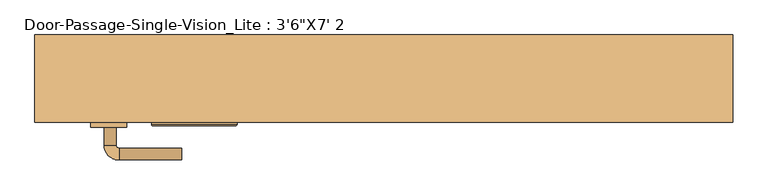
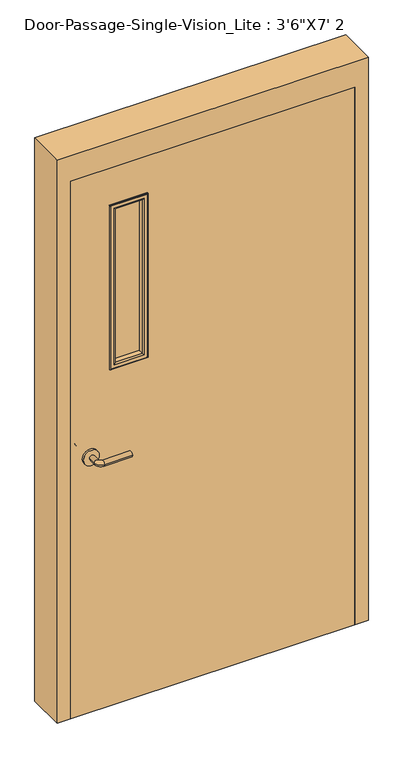
"""IFC4 building model written with IfcOpenShell, lengths in millimetres: door geometry."""

from ifc_helpers import new_model, si_unit, point, frame, frame_2d, origin, place, context, project, spatial, polyline, circle_curve, ellipse_curve, trimmed, segment, composite_curve, outline, extrude, faceted_brep, source, transform, mapped, element, save
from ifc_brep_helpers import plane_surface, cylinder_surface, revolved_surface, advanced_brep


def door_4f5842df(model_context):
    return source(origin(), model_context, "Body", "SolidModel", [
        advanced_brep(
        [(-468.390625, 14.35, 1016.0), (-448.390625, 14.35, 1016.0), (-468.390625, 44.35, 1016.0), (-448.390625, 44.35, 1016.0), (-443.390625, 49.35, 1016.0), (-443.390625, 69.35, 1016.0), (-338.390625, 69.35, 1016.0), (-338.390625, 49.35, 1016.0)],
        [
            (0, 1, circle_curve(frame((-458.390625, 14.35, 1016.0), z_axis=(0.0, -1.0, 0.0), x_axis=(1.0, 0.0, 0.0)), 10.0)),
            (1, 0, circle_curve(frame((-458.390625, 14.35, 1016.0), z_axis=(0.0, -1.0, 0.0), x_axis=(1.0, 0.0, 0.0)), 10.0)),
            (0, 2),
            (2, 3, circle_curve(frame((-458.390625, 44.35, 1016.0), z_axis=(0.0, -1.0, 0.0), x_axis=(1.0, 0.0, 0.0)), 10.0)),
            (3, 1),
            (3, 2, circle_curve(frame((-458.390625, 44.35, 1016.0), z_axis=(0.0, -1.0, 0.0), x_axis=(1.0, 0.0, 0.0)), 10.0)),
            (4, 3, circle_curve(frame((-443.390625, 44.35, 1016.0), z_axis=(0.0, 0.0, 1.0), x_axis=(-1.0, 0.0, 0.0)), 5.0)),
            (2, 5, circle_curve(frame((-443.390625, 44.35, 1016.0), z_axis=(0.0, 0.0, -1.0), x_axis=(-1.0, 0.0, 0.0)), 25.0)),
            (5, 4, circle_curve(frame((-443.390625, 59.35, 1016.0), z_axis=(-1.0, 0.0, 0.0), x_axis=(0.0, -1.0, 0.0)), 10.0)),
            (4, 5, circle_curve(frame((-443.390625, 59.35, 1016.0), z_axis=(-1.0, 0.0, 0.0), x_axis=(0.0, -1.0, 0.0)), 10.0)),
            (6, 7, circle_curve(frame((-338.390625, 59.35, 1016.0), z_axis=(1.0, 0.0, 0.0), x_axis=(0.0, -1.0, 0.0)), 10.0)),
            (7, 6, circle_curve(frame((-338.390625, 59.35, 1016.0), z_axis=(1.0, 0.0, 0.0), x_axis=(0.0, -1.0, 0.0)), 10.0)),
            (5, 6),
            (7, 4),
        ],
        [
            plane_surface(frame((-458.390625, 14.35, 1016.0), z_axis=(0.0, -1.0, 0.0), x_axis=(0.0, 0.0, 1.0))),
            cylinder_surface(frame((-458.390625, 14.35, 1016.0), z_axis=(0.0, -1.0, 0.0), x_axis=(1.0, 0.0, 0.0)), 10.0),
            revolved_surface(trimmed(ellipse_curve(frame((-458.390625, 44.35, 1016.0), z_axis=(0.0, -1.0, 0.0), x_axis=(1.0, 0.0, 0.0)), 10.0, 10.0), [point((-468.390625, 44.35, 1016.0))], [point((-448.390625, 44.35, 1016.0))], True, "CARTESIAN"), (-443.390625, 44.35, 1016.0), (0.0, 0.0, -1.0)),
            revolved_surface(trimmed(ellipse_curve(frame((-458.390625, 44.35, 1016.0), z_axis=(0.0, -1.0, 0.0), x_axis=(1.0, 0.0, 0.0)), 10.0, 10.0), [point((-448.390625, 44.35, 1016.0))], [point((-468.390625, 44.35, 1016.0))], True, "CARTESIAN"), (-443.390625, 44.35, 1016.0), (0.0, 0.0, -1.0)),
            plane_surface(frame((-338.390625, 59.35, 1016.0), z_axis=(1.0, 0.0, 0.0), x_axis=(0.0, 0.0, 1.0))),
            cylinder_surface(frame((-443.390625, 59.35, 1016.0), z_axis=(-1.0, 0.0, 0.0), x_axis=(0.0, -1.0, 0.0)), 10.0),
        ],
        [
            (0, [[1, 2]]),
            (1, [[-1, 3, 4, 5]]),
            (1, [[-2, -5, 6, -3]]),
            (2, [[7, -4, 8, 9]]),
            (3, [[-8, -6, -7, 10]]),
            (4, [[11, 12]]),
            (5, [[-9, 13, -12, 14]]),
            (5, [[-10, -14, -11, -13]]),
        ],
    ),
        extrude(outline(composite_curve([segment(trimmed(circle_curve(frame_2d((1016.0, -460.890625)), 30.0), [point((1016.0, -490.890625))], [point((1016.0, -430.890625))], False, "CARTESIAN"), True, "CONTINUOUS"), segment(trimmed(circle_curve(frame_2d((1016.0, -460.890625)), 30.0), [point((1016.0, -430.890625))], [point((1016.0, -490.890625))], False, "CARTESIAN"), True, "CONTINUOUS")], self_intersect=False)), frame((0.0, 6.35, 0.0), z_axis=(0.0, 1.0, 0.0), x_axis=(0.0, 0.0, 1.0)), (0.0, 0.0, 1.0), 8.0),
        advanced_brep(
        [(-468.390625, -46.1, 1016.0), (-448.390625, -46.1, 1016.0), (-448.390625, -76.1, 1016.0), (-468.390625, -76.1, 1016.0), (-443.390625, -81.1, 1016.0), (-443.390625, -101.1, 1016.0), (-338.390625, -101.1, 1016.0), (-338.390625, -81.1, 1016.0)],
        [
            (0, 1, circle_curve(frame((-458.390625, -46.1, 1016.0), z_axis=(0.0, 1.0, 0.0), x_axis=(1.0, 0.0, 0.0)), 10.0)),
            (1, 0, circle_curve(frame((-458.390625, -46.1, 1016.0), z_axis=(0.0, 1.0, 0.0), x_axis=(1.0, 0.0, 0.0)), 10.0)),
            (1, 2),
            (2, 3, circle_curve(frame((-458.390625, -76.1, 1016.0), z_axis=(0.0, 1.0, 0.0), x_axis=(1.0, 0.0, 0.0)), 10.0)),
            (3, 0),
            (3, 2, circle_curve(frame((-458.390625, -76.1, 1016.0), z_axis=(0.0, 1.0, 0.0), x_axis=(1.0, 0.0, 0.0)), 10.0)),
            (4, 5, circle_curve(frame((-443.390625, -91.1, 1016.0), z_axis=(-1.0, 0.0, 0.0), x_axis=(0.0, 1.0, 0.0)), 10.0)),
            (5, 3, circle_curve(frame((-443.390625, -76.1, 1016.0), z_axis=(0.0, 0.0, -1.0), x_axis=(-1.0, 0.0, 0.0)), 25.0)),
            (2, 4, circle_curve(frame((-443.390625, -76.1, 1016.0), z_axis=(0.0, 0.0, 1.0), x_axis=(-1.0, 0.0, 0.0)), 5.0)),
            (5, 4, circle_curve(frame((-443.390625, -91.1, 1016.0), z_axis=(-1.0, 0.0, 0.0), x_axis=(0.0, 1.0, 0.0)), 10.0)),
            (6, 7, circle_curve(frame((-338.390625, -91.1, 1016.0), z_axis=(1.0, 0.0, 0.0), x_axis=(0.0, 1.0, 0.0)), 10.0)),
            (7, 6, circle_curve(frame((-338.390625, -91.1, 1016.0), z_axis=(1.0, 0.0, 0.0), x_axis=(0.0, 1.0, 0.0)), 10.0)),
            (4, 7),
            (6, 5),
        ],
        [
            plane_surface(frame((-458.390625, -46.1, 1016.0), z_axis=(0.0, 1.0, 0.0), x_axis=(0.0, 0.0, 1.0))),
            cylinder_surface(frame((-458.390625, -46.1, 1016.0), z_axis=(0.0, 1.0, 0.0), x_axis=(1.0, 0.0, 0.0)), 10.0),
            revolved_surface(trimmed(ellipse_curve(frame((-458.390625, -76.1, 1016.0), z_axis=(0.0, -1.0, 0.0), x_axis=(1.0, 0.0, 0.0)), 10.0, 10.0), [point((-468.390625, -76.1, 1016.0))], [point((-448.390625, -76.1, 1016.0))], True, "CARTESIAN"), (-443.390625, -76.1, 1016.0), (0.0, 0.0, -1.0)),
            revolved_surface(trimmed(ellipse_curve(frame((-458.390625, -76.1, 1016.0), z_axis=(0.0, -1.0, 0.0), x_axis=(1.0, 0.0, 0.0)), 10.0, 10.0), [point((-448.390625, -76.1, 1016.0))], [point((-468.390625, -76.1, 1016.0))], True, "CARTESIAN"), (-443.390625, -76.1, 1016.0), (0.0, 0.0, -1.0)),
            plane_surface(frame((-338.390625, -91.1, 1016.0), z_axis=(1.0, 0.0, 0.0), x_axis=(0.0, 0.0, 1.0))),
            cylinder_surface(frame((-443.390625, -91.1, 1016.0), z_axis=(-1.0, 0.0, 0.0), x_axis=(0.0, 1.0, 0.0)), 10.0),
        ],
        [
            (0, [[1, 2]]),
            (1, [[3, 4, 5, -2]]),
            (1, [[-5, 6, -3, -1]]),
            (2, [[7, 8, -4, 9]]),
            (3, [[10, -9, -6, -8]]),
            (4, [[11, 12]]),
            (5, [[13, -11, 14, -7]]),
            (5, [[-14, -12, -13, -10]]),
        ],
    ),
        extrude(outline(composite_curve([segment(trimmed(circle_curve(frame_2d((1016.0, -460.890625)), 30.0), [point((1016.0, -490.890625))], [point((1016.0, -430.890625))], False, "CARTESIAN"), True, "CONTINUOUS"), segment(trimmed(circle_curve(frame_2d((1016.0, -460.890625)), 30.0), [point((1016.0, -430.890625))], [point((1016.0, -490.890625))], False, "CARTESIAN"), True, "CONTINUOUS")], self_intersect=False)), frame((0.0, -46.1, 0.0), z_axis=(0.0, 1.0, 0.0), x_axis=(0.0, 0.0, 1.0)), (0.0, 0.0, 1.0), 8.0),
        extrude(outline(polyline([(2133.6, -533.4), (0.0, -533.4), (0.0, 533.4), (2133.6, 533.4), (2133.6, -533.4)]), holes=[polyline([(1981.2, -381.0), (1981.2, -254.0), (1346.2, -254.0), (1346.2, -381.0), (1981.2, -381.0)])]), frame((0.0, -38.1, 0.0), z_axis=(0.0, 1.0, 0.0), x_axis=(0.0, 0.0, 1.0)), (0.0, 0.0, 1.0), 44.45),
        faceted_brep([(533.4, 11.1125, 0.0), (517.525, 11.1125, 0.0), (517.525, 58.7375, 0.0), (533.4, 58.7375, 0.0), (533.4, 107.95, 0.0), (584.2, 107.95, 0.0), (584.2, -38.1, 0.0), (533.4, -38.1, 0.0), (533.4, -38.1, 2133.6), (533.4, 11.1125, 2133.6), (584.2, -38.1, 2235.2), (-584.2, -38.1, 2235.2), (-584.2, -38.1, 0.0), (-533.4, -38.1, 0.0), (-533.4, -38.1, 2133.6), (584.2, 107.95, 2235.2), (533.4, 107.95, 2133.6), (-533.4, 107.95, 2133.6), (-533.4, 107.95, 0.0), (-584.2, 107.95, 0.0), (-584.2, 107.95, 2235.2), (533.4, 58.7375, 2133.6), (517.525, 58.7375, 2117.725), (-517.525, 58.7375, 2117.725), (-517.525, 58.7375, 0.0), (-533.4, 58.7375, 0.0), (-533.4, 58.7375, 2133.6), (517.525, 11.1125, 2117.725), (-533.4, 11.1125, 2133.6), (-533.4, 11.1125, 0.0), (-517.525, 11.1125, 0.0), (-517.525, 11.1125, 2117.725)], [[[0, 1, 2, 3, 4, 5, 6, 7]], [[7, 8, 9, 0]], [[6, 10, 11, 12, 13, 14, 8, 7]], [[5, 15, 10, 6]], [[4, 16, 17, 18, 19, 20, 15, 5]], [[3, 21, 16, 4]], [[2, 22, 23, 24, 25, 26, 21, 3]], [[1, 27, 22, 2]], [[0, 9, 28, 29, 30, 31, 27, 1]], [[8, 14, 28, 9]], [[16, 21, 26, 17]], [[22, 27, 31, 23]], [[12, 19, 18, 25, 24, 30, 29, 13]], [[13, 29, 28, 14]], [[11, 20, 19, 12]], [[17, 26, 25, 18]], [[23, 31, 30, 24]], [[15, 20, 11, 10]]]),
        extrude(outline(polyline([(-254.0, -12.7), (-254.0, -19.05), (-381.0, -19.05), (-381.0, -12.7), (-254.0, -12.7)])), frame((0.0, 0.0, 1346.2), z_axis=(0.0, 0.0, 1.0), x_axis=(1.0, 0.0, 0.0)), (0.0, 0.0, 1.0), 635.0),
        advanced_brep(
        [(-381.0, -19.05, 1981.2), (-381.0, -19.05, 1346.2), (-381.0, -38.1, 1346.2), (-381.0, -38.1, 1981.2), (-369.0, -39.1, 1969.2), (-369.0, -39.1, 1358.2), (-369.0, -19.05, 1358.2), (-369.0, -19.05, 1969.2), (-374.0, -44.1, 1974.2), (-374.0, -44.1, 1353.2), (-389.0, -42.1, 1989.2), (-389.0, -42.1, 1338.2), (-387.0, -44.1, 1340.2), (-387.0, -44.1, 1987.2), (-389.0, -38.1, 1989.2), (-389.0, -38.1, 1338.2), (-254.0, -19.05, 1346.2), (-254.0, -38.1, 1346.2), (-266.0, -39.1, 1358.2), (-266.0, -19.05, 1358.2), (-261.0, -44.1, 1353.2), (-246.0, -42.1, 1338.2), (-248.0, -44.1, 1340.2), (-246.0, -38.1, 1338.2), (-254.0, -19.05, 1981.2), (-254.0, -38.1, 1981.2), (-266.0, -39.1, 1969.2), (-266.0, -19.05, 1969.2), (-261.0, -44.1, 1974.2), (-246.0, -42.1, 1989.2), (-248.0, -44.1, 1987.2), (-246.0, -38.1, 1989.2)],
        [
            (0, 1),
            (1, 2),
            (2, 3),
            (3, 0),
            (4, 5),
            (5, 6),
            (6, 7),
            (7, 4),
            (8, 9),
            (9, 5, ellipse_curve(frame((-374.0, -39.1, 1353.2), z_axis=(-0.7071067811865475, 0.0, 0.7071067811865475), x_axis=(0.7071067811865474, 0.0, 0.7071067811865476)), 7.0710678, 5.0)),
            (4, 8, ellipse_curve(frame((-374.0, -39.1, 1974.2), z_axis=(-0.7071067811865475, 0.0, -0.7071067811865475), x_axis=(-0.7071067811865474, 0.0, 0.7071067811865476)), 7.0710678, 5.0)),
            (10, 11),
            (11, 12, ellipse_curve(frame((-387.0, -42.1, 1340.2), z_axis=(-0.7071067811865475, 0.0, 0.7071067811865475), x_axis=(0.7071067811865474, 0.0, 0.7071067811865476)), 2.8284271, 2.0)),
            (12, 13),
            (13, 10, ellipse_curve(frame((-387.0, -42.1, 1987.2), z_axis=(-0.7071067811865475, 0.0, -0.7071067811865475), x_axis=(-0.7071067811865474, 0.0, 0.7071067811865476)), 2.8284271, 2.0)),
            (14, 15),
            (15, 11),
            (10, 14),
            (1, 16),
            (16, 17),
            (17, 2),
            (5, 18),
            (18, 19),
            (19, 6),
            (9, 20),
            (20, 18, ellipse_curve(frame((-261.0, -39.1, 1353.2), z_axis=(-0.7071067811865475, 0.0, -0.7071067811865475), x_axis=(-0.7071067811865476, 0.0, 0.7071067811865474)), 7.0710678, 5.0)),
            (11, 21),
            (21, 22, ellipse_curve(frame((-248.0, -42.1, 1340.2), z_axis=(-0.7071067811865475, 0.0, -0.7071067811865475), x_axis=(-0.7071067811865476, 0.0, 0.7071067811865474)), 2.8284271, 2.0)),
            (22, 12),
            (15, 23),
            (23, 21),
            (16, 24),
            (24, 25),
            (25, 17),
            (18, 26),
            (26, 27),
            (27, 19),
            (20, 28),
            (28, 26, ellipse_curve(frame((-261.0, -39.1, 1974.2), z_axis=(0.7071067811865475, 0.0, -0.7071067811865475), x_axis=(-0.7071067811865474, 0.0, -0.7071067811865476)), 7.0710678, 5.0)),
            (21, 29),
            (29, 30, ellipse_curve(frame((-248.0, -42.1, 1987.2), z_axis=(0.7071067811865475, 0.0, -0.7071067811865475), x_axis=(-0.7071067811865474, 0.0, -0.7071067811865476)), 2.8284271, 2.0)),
            (30, 22),
            (23, 31),
            (31, 29),
            (14, 31),
            (25, 3),
            (24, 0),
            (27, 7),
            (26, 4),
            (28, 8),
            (30, 13),
            (29, 10),
        ],
        [
            plane_surface(frame((-381.0, -38.1, 1981.2), z_axis=(-1.0, 0.0, 0.0), x_axis=(0.0, 0.0, -1.0))),
            plane_surface(frame((-369.0, -19.05, 1969.2), z_axis=(1.0, 0.0, 0.0), x_axis=(0.0, 0.0, -1.0))),
            cylinder_surface(frame((-374.0, -39.1, 1981.2), z_axis=(0.0, 0.0, 1.0), x_axis=(-1.0, 0.0, 0.0)), 5.0),
            cylinder_surface(frame((-387.0, -42.1, 1981.2), z_axis=(0.0, 0.0, 1.0), x_axis=(-1.0, 0.0, 0.0)), 2.0),
            plane_surface(frame((-389.0, -42.1, 1989.2), z_axis=(-1.0, 0.0, 0.0), x_axis=(0.0, 0.0, -1.0))),
            plane_surface(frame((-381.0, -38.1, 1346.2), z_axis=(0.0, 0.0, -1.0), x_axis=(1.0, 0.0, 0.0))),
            plane_surface(frame((-369.0, -19.05, 1358.2), z_axis=(0.0, 0.0, 1.0), x_axis=(1.0, 0.0, 0.0))),
            cylinder_surface(frame((-381.0, -39.1, 1353.2), z_axis=(-1.0, 0.0, 0.0), x_axis=(0.0, 0.0, -1.0)), 5.0),
            cylinder_surface(frame((-381.0, -42.1, 1340.2), z_axis=(-1.0, 0.0, 0.0), x_axis=(0.0, 0.0, -1.0)), 2.0),
            plane_surface(frame((-389.0, -42.1, 1338.2), z_axis=(0.0, 0.0, -1.0), x_axis=(1.0, 0.0, 0.0))),
            plane_surface(frame((-254.0, -38.1, 1346.2), z_axis=(1.0, 0.0, 0.0), x_axis=(0.0, 0.0, 1.0))),
            plane_surface(frame((-266.0, -19.05, 1358.2), z_axis=(-1.0, 0.0, 0.0), x_axis=(0.0, 0.0, 1.0))),
            cylinder_surface(frame((-261.0, -39.1, 1346.2), z_axis=(0.0, 0.0, -1.0), x_axis=(1.0, 0.0, 0.0)), 5.0),
            cylinder_surface(frame((-248.0, -42.1, 1346.2), z_axis=(0.0, 0.0, -1.0), x_axis=(1.0, 0.0, 0.0)), 2.0),
            plane_surface(frame((-246.0, -42.1, 1338.2), z_axis=(1.0, 0.0, 0.0), x_axis=(0.0, 0.0, 1.0))),
            plane_surface(frame((-246.0, -38.1, 1989.2), z_axis=(0.0, 1.0, 0.0), x_axis=(-1.0, 0.0, 0.0))),
            plane_surface(frame((-254.0, -38.1, 1981.2), z_axis=(0.0, 0.0, 1.0), x_axis=(-1.0, 0.0, 0.0))),
            plane_surface(frame((-254.0, -19.05, 1981.2), z_axis=(0.0, 1.0, 0.0), x_axis=(-1.0, 0.0, 0.0))),
            plane_surface(frame((-266.0, -19.05, 1969.2), z_axis=(0.0, 0.0, -1.0), x_axis=(-1.0, 0.0, 0.0))),
            cylinder_surface(frame((-254.0, -39.1, 1974.2), z_axis=(1.0, 0.0, 0.0), x_axis=(0.0, 0.0, 1.0)), 5.0),
            plane_surface(frame((-261.0, -44.1, 1974.2), z_axis=(0.0, -1.0, 0.0), x_axis=(-1.0, 0.0, 0.0))),
            cylinder_surface(frame((-254.0, -42.1, 1987.2), z_axis=(1.0, 0.0, 0.0), x_axis=(0.0, 0.0, 1.0)), 2.0),
            plane_surface(frame((-246.0, -42.1, 1989.2), z_axis=(0.0, 0.0, 1.0), x_axis=(-1.0, 0.0, 0.0))),
        ],
        [
            (0, [[1, 2, 3, 4]]),
            (1, [[5, 6, 7, 8]]),
            (2, [[9, 10, -5, 11]]),
            (3, [[12, 13, 14, 15]]),
            (4, [[16, 17, -12, 18]]),
            (5, [[19, 20, 21, -2]]),
            (6, [[22, 23, 24, -6]]),
            (7, [[25, 26, -22, -10]]),
            (8, [[27, 28, 29, -13]]),
            (9, [[30, 31, -27, -17]]),
            (10, [[32, 33, 34, -20]]),
            (11, [[35, 36, 37, -23]]),
            (12, [[38, 39, -35, -26]]),
            (13, [[40, 41, 42, -28]]),
            (14, [[43, 44, -40, -31]]),
            (15, [[-16, 45, -43, -30], [-3, -21, -34, 46]]),
            (16, [[47, -4, -46, -33]]),
            (17, [[-1, -47, -32, -19], [-7, -24, -37, 48]]),
            (18, [[49, -8, -48, -36]]),
            (19, [[50, -11, -49, -39]]),
            (20, [[-14, -29, -42, 51], [-9, -50, -38, -25]]),
            (21, [[52, -15, -51, -41]]),
            (22, [[-45, -18, -52, -44]]),
        ],
    ),
        advanced_brep(
        [(-381.0, -12.7, 1346.2), (-381.0, -12.7, 1981.2), (-381.0, 6.35, 1981.2), (-381.0, 6.35, 1346.2), (-369.0, 7.35, 1358.2), (-369.0, 7.35, 1969.2), (-369.0, -12.7, 1969.2), (-369.0, -12.7, 1358.2), (-374.0, 12.35, 1353.2), (-374.0, 12.35, 1974.2), (-389.0, 10.35, 1338.2), (-389.0, 10.35, 1989.2), (-387.0, 12.35, 1987.2), (-387.0, 12.35, 1340.2), (-389.0, 6.35, 1338.2), (-389.0, 6.35, 1989.2), (-254.0, -12.7, 1981.2), (-254.0, 6.35, 1981.2), (-266.0, 7.35, 1969.2), (-266.0, -12.7, 1969.2), (-261.0, 12.35, 1974.2), (-246.0, 10.35, 1989.2), (-248.0, 12.35, 1987.2), (-246.0, 6.35, 1989.2), (-254.0, -12.7, 1346.2), (-254.0, 6.35, 1346.2), (-266.0, 7.35, 1358.2), (-266.0, -12.7, 1358.2), (-261.0, 12.35, 1353.2), (-246.0, 10.35, 1338.2), (-248.0, 12.35, 1340.2), (-246.0, 6.35, 1338.2)],
        [
            (0, 1),
            (1, 2),
            (2, 3),
            (3, 0),
            (4, 5),
            (5, 6),
            (6, 7),
            (7, 4),
            (8, 9),
            (9, 5, ellipse_curve(frame((-374.0, 7.35, 1974.2), z_axis=(-0.7071067811865475, 0.0, -0.7071067811865475), x_axis=(0.7071067811865474, 0.0, -0.7071067811865476)), 7.0710678, 5.0)),
            (4, 8, ellipse_curve(frame((-374.0, 7.35, 1353.2), z_axis=(-0.7071067811865475, 0.0, 0.7071067811865475), x_axis=(-0.7071067811865474, 0.0, -0.7071067811865476)), 7.0710678, 5.0)),
            (10, 11),
            (11, 12, ellipse_curve(frame((-387.0, 10.35, 1987.2), z_axis=(-0.7071067811865475, 0.0, -0.7071067811865475), x_axis=(0.7071067811865474, 0.0, -0.7071067811865476)), 2.8284271, 2.0)),
            (12, 13),
            (13, 10, ellipse_curve(frame((-387.0, 10.35, 1340.2), z_axis=(-0.7071067811865475, 0.0, 0.7071067811865475), x_axis=(-0.7071067811865474, 0.0, -0.7071067811865476)), 2.8284271, 2.0)),
            (14, 15),
            (15, 11),
            (10, 14),
            (1, 16),
            (16, 17),
            (17, 2),
            (5, 18),
            (18, 19),
            (19, 6),
            (9, 20),
            (20, 18, ellipse_curve(frame((-261.0, 7.35, 1974.2), z_axis=(-0.7071067811865475, 0.0, 0.7071067811865475), x_axis=(-0.7071067811865476, 0.0, -0.7071067811865474)), 7.0710678, 5.0)),
            (11, 21),
            (21, 22, ellipse_curve(frame((-248.0, 10.35, 1987.2), z_axis=(-0.7071067811865475, 0.0, 0.7071067811865475), x_axis=(-0.7071067811865476, 0.0, -0.7071067811865474)), 2.8284271, 2.0)),
            (22, 12),
            (15, 23),
            (23, 21),
            (16, 24),
            (24, 25),
            (25, 17),
            (18, 26),
            (26, 27),
            (27, 19),
            (20, 28),
            (28, 26, ellipse_curve(frame((-261.0, 7.35, 1353.2), z_axis=(0.7071067811865475, 0.0, 0.7071067811865475), x_axis=(-0.7071067811865474, 0.0, 0.7071067811865476)), 7.0710678, 5.0)),
            (21, 29),
            (29, 30, ellipse_curve(frame((-248.0, 10.35, 1340.2), z_axis=(0.7071067811865475, 0.0, 0.7071067811865475), x_axis=(-0.7071067811865474, 0.0, 0.7071067811865476)), 2.8284271, 2.0)),
            (30, 22),
            (23, 31),
            (31, 29),
            (14, 31),
            (25, 3),
            (24, 0),
            (27, 7),
            (26, 4),
            (28, 8),
            (30, 13),
            (29, 10),
        ],
        [
            plane_surface(frame((-381.0, 6.35, 1346.2), z_axis=(-1.0, 0.0, 0.0), x_axis=(0.0, 0.0, 1.0))),
            plane_surface(frame((-369.0, -12.7, 1358.2), z_axis=(1.0, 0.0, 0.0), x_axis=(0.0, 0.0, 1.0))),
            cylinder_surface(frame((-374.0, 7.35, 1346.2), z_axis=(0.0, 0.0, -1.0), x_axis=(-1.0, 0.0, 0.0)), 5.0),
            cylinder_surface(frame((-387.0, 10.35, 1346.2), z_axis=(0.0, 0.0, -1.0), x_axis=(-1.0, 0.0, 0.0)), 2.0),
            plane_surface(frame((-389.0, 10.35, 1338.2), z_axis=(-1.0, 0.0, 0.0), x_axis=(0.0, 0.0, 1.0))),
            plane_surface(frame((-381.0, 6.35, 1981.2), z_axis=(0.0, 0.0, 1.0), x_axis=(1.0, 0.0, 0.0))),
            plane_surface(frame((-369.0, -12.7, 1969.2), z_axis=(0.0, 0.0, -1.0), x_axis=(1.0, 0.0, 0.0))),
            cylinder_surface(frame((-381.0, 7.35, 1974.2), z_axis=(-1.0, 0.0, 0.0), x_axis=(0.0, 0.0, 1.0)), 5.0),
            cylinder_surface(frame((-381.0, 10.35, 1987.2), z_axis=(-1.0, 0.0, 0.0), x_axis=(0.0, 0.0, 1.0)), 2.0),
            plane_surface(frame((-389.0, 10.35, 1989.2), z_axis=(0.0, 0.0, 1.0), x_axis=(1.0, 0.0, 0.0))),
            plane_surface(frame((-254.0, 6.35, 1981.2), z_axis=(1.0, 0.0, 0.0), x_axis=(0.0, 0.0, -1.0))),
            plane_surface(frame((-266.0, -12.7, 1969.2), z_axis=(-1.0, 0.0, 0.0), x_axis=(0.0, 0.0, -1.0))),
            cylinder_surface(frame((-261.0, 7.35, 1981.2), z_axis=(0.0, 0.0, 1.0), x_axis=(1.0, 0.0, 0.0)), 5.0),
            cylinder_surface(frame((-248.0, 10.35, 1981.2), z_axis=(0.0, 0.0, 1.0), x_axis=(1.0, 0.0, 0.0)), 2.0),
            plane_surface(frame((-246.0, 10.35, 1989.2), z_axis=(1.0, 0.0, 0.0), x_axis=(0.0, 0.0, -1.0))),
            plane_surface(frame((-246.0, 6.35, 1338.2), z_axis=(0.0, -1.0, 0.0), x_axis=(-1.0, 0.0, 0.0))),
            plane_surface(frame((-254.0, 6.35, 1346.2), z_axis=(0.0, 0.0, -1.0), x_axis=(-1.0, 0.0, 0.0))),
            plane_surface(frame((-254.0, -12.7, 1346.2), z_axis=(0.0, -1.0, 0.0), x_axis=(-1.0, 0.0, 0.0))),
            plane_surface(frame((-266.0, -12.7, 1358.2), z_axis=(0.0, 0.0, 1.0), x_axis=(-1.0, 0.0, 0.0))),
            cylinder_surface(frame((-254.0, 7.35, 1353.2), z_axis=(1.0, 0.0, 0.0), x_axis=(0.0, 0.0, -1.0)), 5.0),
            plane_surface(frame((-261.0, 12.35, 1353.2), z_axis=(0.0, 1.0, 0.0), x_axis=(-1.0, 0.0, 0.0))),
            cylinder_surface(frame((-254.0, 10.35, 1340.2), z_axis=(1.0, 0.0, 0.0), x_axis=(0.0, 0.0, -1.0)), 2.0),
            plane_surface(frame((-246.0, 10.35, 1338.2), z_axis=(0.0, 0.0, -1.0), x_axis=(-1.0, 0.0, 0.0))),
        ],
        [
            (0, [[1, 2, 3, 4]]),
            (1, [[5, 6, 7, 8]]),
            (2, [[9, 10, -5, 11]]),
            (3, [[12, 13, 14, 15]]),
            (4, [[16, 17, -12, 18]]),
            (5, [[19, 20, 21, -2]]),
            (6, [[22, 23, 24, -6]]),
            (7, [[25, 26, -22, -10]]),
            (8, [[27, 28, 29, -13]]),
            (9, [[30, 31, -27, -17]]),
            (10, [[32, 33, 34, -20]]),
            (11, [[35, 36, 37, -23]]),
            (12, [[38, 39, -35, -26]]),
            (13, [[40, 41, 42, -28]]),
            (14, [[43, 44, -40, -31]]),
            (15, [[-16, 45, -43, -30], [-3, -21, -34, 46]]),
            (16, [[47, -4, -46, -33]]),
            (17, [[-1, -47, -32, -19], [-7, -24, -37, 48]]),
            (18, [[49, -8, -48, -36]]),
            (19, [[50, -11, -49, -39]]),
            (20, [[-14, -29, -42, 51], [-9, -50, -38, -25]]),
            (21, [[52, -15, -51, -41]]),
            (22, [[-45, -18, -52, -44]]),
        ],
    ),
    ])


if __name__ == "__main__":
    model = new_model("IFC4")
    model_context = context("Model", 3, world=origin())
    ifc_project = project(units=[si_unit("LENGTHUNIT", "METRE", prefix="MILLI")], contexts=[model_context])
    site = spatial("IfcSite", under=ifc_project)
    building = spatial("IfcBuilding", under=site)
    placement = place(None, origin())
    door_shape = door_4f5842df(model_context)
    element("IfcDoor", 1, ObjectType="Door-Passage-Single-Vision_Lite : 3'6\"X7' 2", at=placement, inside=building, context=model_context, shape_type="MappedRepresentation", body=[
        mapped(door_shape, transform((0.0, 0.0, 0.0), x_axis=(1.0, 0.0, 0.0), y_axis=(0.0, 1.0, 0.0), z_axis=(0.0, 0.0, 1.0))),
    ])
    save(model, "model.ifc")

# Revit data of these elements
# Type "Door-Passage-Single-Vision_Lite : 3'6\"X7' 2"
#   Type Mark = "14"
#   Assembly Code = "B2030100"
#   Analytic Construction = "Wooden"
#   Thickness = 0' - 1 3/4"
#   Thermal Resistance (R) = 2.5876 (h·ft²·°F)/BTU
#   Swing Angle [instance default] = 90.00°
#   Strike Height = 3' - 4"
#   Rough Width [instance default] = 3' - 10"
#   Rough Height [instance default] = 7' - 4"
#   MFOpeningHeight [instance default] = 0' - 4"
#   MFOpeningWidth [instance default] = 0' - 4"
#   Inset Calculate [instance default] = 0' - 4"
#   Masonry Inset [instance default] = 0' - 1"
#   Height = 7' - 0"
#   Width = 3' - 6"
#   Heat Transfer Coefficient (U) = 0.3865 BTU/(h·ft²·°F)
#   Masonry Frame Depth = 0' - 5 3/4"
#   Masonry Frame [instance default] = yes
#   Function = 1
#   Dry Wall Frame [instance default] = no
#   Panel Material = Wood - Birch
#   Glazing = Glass
#   Glass Stop Material = Metal - Paint Finish - Grey
#   Frame Material = Metal - Paint Finish - Grey
#   Door Handle Material = Aluminum
#   Visual Light Transmittance = 0
#   Solar Heat Gain Coefficient = 0
#   Wall Closure = (empty or 0)
# Element 1 (IfcDoor, "Door-Passage-Single-Vision_Lite : 3'6\"X7' 2")
#   Materials on its faces: "Metal - Paint Finish - Grey", "Aluminum", "Wood - Birch", "Glass"
# Materials
#   "Wood - Birch": class "Wood", colour RGB 166 116 52, transparency 0, Cost = 0
#   "Glass": class "Glass", colour RGB 0 128 192, transparency 0.75, Description = "Soda Lime Glass", Cost = 0
#   "Metal - Paint Finish - Grey": class "Paint", colour RGB 104 104 104, transparency 0, Cost = 0
#   "Aluminum": class "Metal", colour RGB 247 247 247, transparency 0, Description = "Aluminum 6061", Cost = 0
